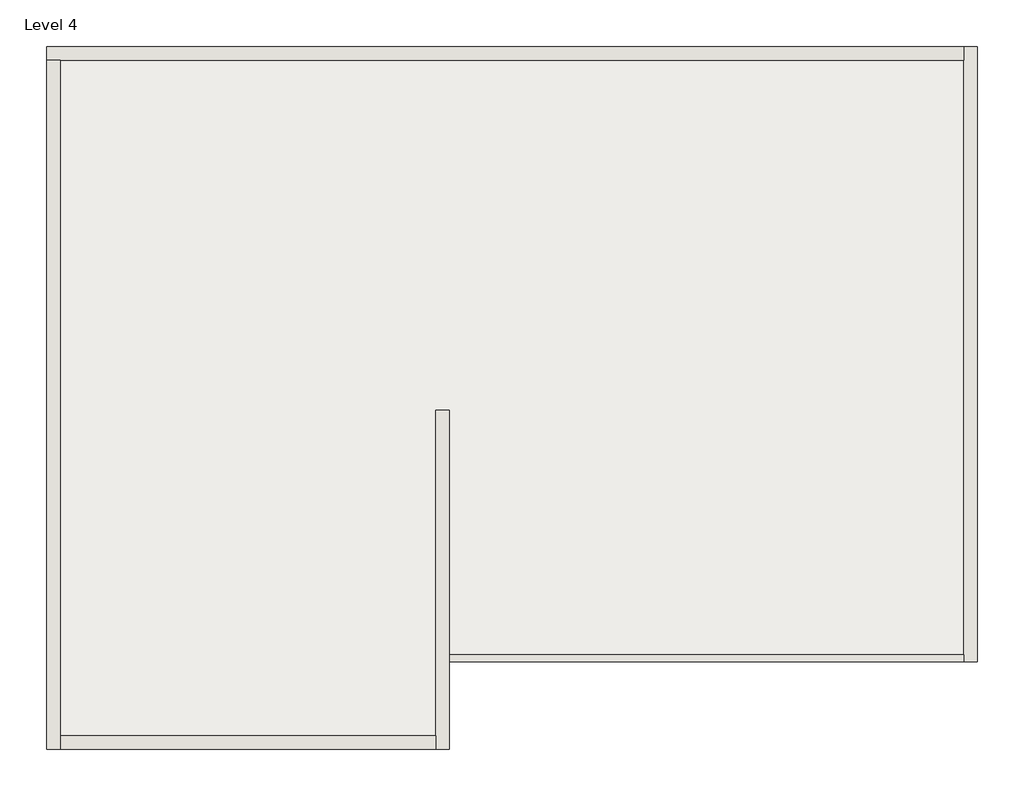
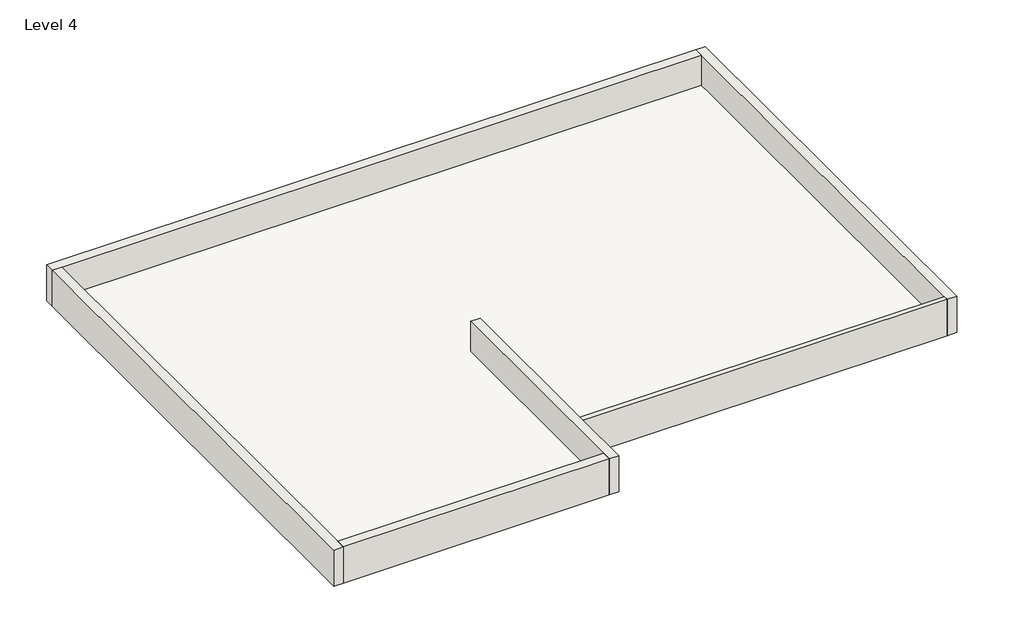
# One storey: 6 walls, 1 roof.
"""IFC4 building model written with IfcOpenShell, lengths in millimetres."""

from ifc_helpers import new_model, si_unit, frame, origin, place, context, project, spatial, polyline, outline, extrude, faceted_brep, element, save

model = new_model("IFC4")

# Units and contexts
model_context = context("Model", 3, world=origin())
ifc_project = project(units=[si_unit("LENGTHUNIT", "METRE", prefix="MILLI")], contexts=[model_context])

# Site, building, storey
site = spatial("IfcSite", under=ifc_project)
building = spatial("IfcBuilding", under=site)
storey = spatial("IfcBuildingStorey", under=building, Name="Level 4", Elevation=6400.8)

# Roof
placement = place(None, origin())
element("IfcRoof", 1, ObjectType="ROOFING 6\"", at=placement, inside=storey, context=model_context, shape_type="SweptSolid", body=[
    extrude(outline(polyline([(-10124.765751, -5996.1053142), (-10124.765751, 5446.5946858), (5178.734249, 5446.5946858), (5178.734249, -4624.5053142), (-3538.1446058, -4624.5053142), (-3538.1446058, -484.3053142), (-3766.7446058, -484.3053142), (-3766.7446058, -5996.1053142), (-10124.765751, -5996.1053142)])), frame((0.0, 0.0, 6400.8), z_axis=(0.0, 0.0, 1.0), x_axis=(1.0, 0.0, 0.0)), (0.0, 0.0, 1.0), 152.4),
])

# Walls
element("IfcWall", 2, at=placement, inside=storey, context=model_context, shape_type="SweptSolid", body=[
    extrude(outline(polyline([(-3766.7446058, -6224.7053142), (-10124.765751, -6224.7053142), (-10124.765751, -5996.1053142), (-3766.7446058, -5996.1053142), (-3766.7446058, -6224.7053142)])), frame((0.0, 0.0, 6400.8), z_axis=(0.0, 0.0, 1.0), x_axis=(1.0, 0.0, 0.0)), (0.0, 0.0, 1.0), 914.4),
])
element("IfcWall", 3, at=placement, inside=storey, context=model_context, shape_type="Brep", body=[
    faceted_brep([(5407.334249, -4738.8053142, 6400.8), (5407.334249, 5675.1946858, 6400.8), (5407.334249, 5675.1946858, 7315.2), (5407.334249, -4738.8053142, 7315.2), (5178.734249, -4738.8053142, 6400.8), (5178.734249, -4738.8053142, 7315.2), (5178.734249, -4624.5053142, 7315.2), (5178.734249, 5446.5946858, 7315.2), (5178.734249, 5675.1946858, 7315.2), (5178.734249, 5675.1946858, 6400.8), (5178.734249, 5446.5946858, 6400.8), (5178.734249, -4624.5053142, 6400.8)], [[[0, 1, 2, 3]], [[4, 5, 6, 7, 8, 9, 10, 11]], [[1, 0, 4, 11, 10, 9]], [[3, 2, 8, 7, 6, 5]], [[2, 1, 9, 8]], [[0, 3, 5, 4]]]),
])
element("IfcWall", 4, at=placement, inside=storey, context=model_context, shape_type="Brep", body=[
    faceted_brep([(5178.734249, 5675.1946858, 6400.8), (-10353.365751, 5675.1946858, 6400.8), (-10353.365751, 5675.1946858, 7315.2), (5178.734249, 5675.1946858, 7315.2), (5178.734249, 5446.5946858, 6400.8), (5178.734249, 5446.5946858, 7315.2), (-10124.765751, 5446.5946858, 7315.2), (-10353.365751, 5446.5946858, 7315.2), (-10353.365751, 5446.5946858, 6400.8), (-10124.765751, 5446.5946858, 6400.8)], [[[0, 1, 2, 3]], [[4, 5, 6, 7, 8, 9]], [[1, 0, 4, 9, 8]], [[3, 2, 7, 6, 5]], [[0, 3, 5, 4]], [[2, 1, 8, 7]]]),
])
element("IfcWall", 5, at=placement, inside=storey, context=model_context, shape_type="Brep", body=[
    faceted_brep([(-10353.365751, 5446.5946858, 6400.8), (-10353.365751, -6224.7053142, 6400.8), (-10353.365751, -6224.7053142, 7315.2), (-10353.365751, 5446.5946858, 7315.2), (-10124.765751, 5446.5946858, 6400.8), (-10124.765751, 5446.5946858, 7315.2), (-10124.765751, -5996.1053142, 7315.2), (-10124.765751, -6224.7053142, 7315.2), (-10124.765751, -6224.7053142, 6400.8), (-10124.765751, -5996.1053142, 6400.8)], [[[0, 1, 2, 3]], [[4, 5, 6, 7, 8, 9]], [[1, 0, 4, 9, 8]], [[3, 2, 7, 6, 5]], [[0, 3, 5, 4]], [[2, 1, 8, 7]]]),
])
element("IfcWall", 6, at=placement, inside=storey, context=model_context, shape_type="Brep", body=[
    faceted_brep([(-3538.1446058, -6224.7053142, 6400.8), (-3538.1446058, -4738.8053142, 6400.8), (-3538.1446058, -4624.5053142, 6400.8), (-3538.1446058, -484.3053142, 6400.8), (-3538.1446058, -484.3053142, 7315.2), (-3538.1446058, -4624.5053142, 7315.2), (-3538.1446058, -4738.8053142, 7315.2), (-3538.1446058, -6224.7053142, 7315.2), (-3766.7446058, -6224.7053142, 6400.8), (-3766.7446058, -6224.7053142, 7315.2), (-3766.7446058, -5996.1053142, 7315.2), (-3766.7446058, -484.3053142, 7315.2), (-3766.7446058, -484.3053142, 6400.8), (-3766.7446058, -5996.1053142, 6400.8)], [[[0, 1, 2, 3, 4, 5, 6, 7]], [[8, 9, 10, 11, 12, 13]], [[3, 2, 1, 0, 8, 13, 12]], [[4, 3, 12, 11]], [[7, 6, 5, 4, 11, 10, 9]], [[0, 7, 9, 8]]]),
])
element("IfcWall", 7, ObjectType="INTERIOR WALL THICKNESS 4.5\"", at=placement, inside=storey, context=model_context, shape_type="SweptSolid", body=[
    extrude(outline(polyline([(5178.734249, -4738.8053142), (-3538.1446058, -4738.8053142), (-3538.1446058, -4624.5053142), (5178.734249, -4624.5053142), (5178.734249, -4738.8053142)])), frame((0.0, 0.0, 6400.8), z_axis=(0.0, 0.0, 1.0), x_axis=(1.0, 0.0, 0.0)), (0.0, 0.0, 1.0), 914.4),
])

save(model, "model.ifc")

# Revit data of these elements
# Type "ROOFING 6\""
#   Assembly Code = "B1020"
#   Layers, outside or top first: 0' - 6" "ROOFING" (function 1)
# Type
#   Assembly Code = "B2010"
#   Layers, outside or top first: 0' - 9" "BEIGE COLOUR" (function 1)
# Type "INTERIOR WALL THICKNESS 4.5\""
#   Assembly Code = "B2010"
#   Layers, outside or top first: 0' - 4 1/2" "BEIGE COLOUR" (function 1)
# Element 1 (IfcRoof, "ROOFING 6\"")
#   built-in parameter 1001705 = 21.5 (stored number, unit not read)
#   built-in parameter 1001710 = 33615
#   Phase Created = New Construction
#   Materials on its faces: "ROOFING"
# Elements 2, 4, 5, 6 (IfcWall)
#   Top Offset = 3' - 0"
#   Base Offset = 0' - 0"
#   wall height = 3' - 0"
#   Phase Created = New Construction
#   Base Constraint = Level 4
#   Top Constraint = Level 4
#   Materials on its faces: "BEIGE COLOUR"
# Element 3 (IfcWall)
#   Top Offset = 0' - 0"
#   Base Offset = 0' - 0"
#   Unconnected Height = 3' - 0"
#   wall height = 3' - 0"
#   Phase Created = New Construction
#   Base Constraint = Level 4
#   Materials on its faces: "BEIGE COLOUR"
# Element 7 (IfcWall, "INTERIOR WALL THICKNESS 4.5\"")
#   Top Offset = 0' - 0"
#   Base Offset = 0' - 0"
#   Unconnected Height = 3' - 0"
#   wall height = 3' - 0"
#   Phase Created = New Construction
#   Base Constraint = Level 4
#   Materials on its faces: "BEIGE COLOUR"
# Materials
#   "ROOFING": class "Generic", colour RGB 120 120 120, transparency 0, Cost = 0
#   "BEIGE COLOUR": class "Generic", colour RGB 120 120 120, transparency 0, Cost = 0
